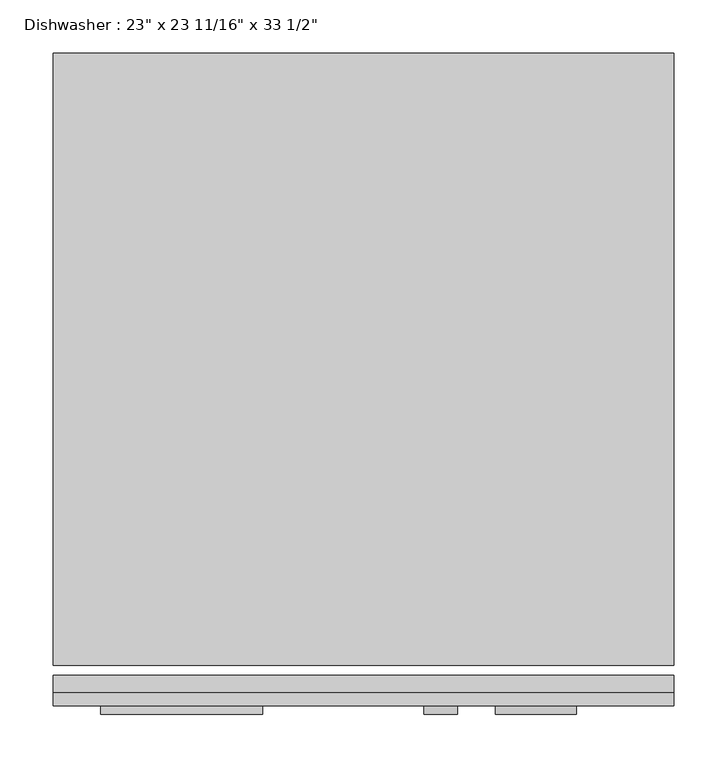
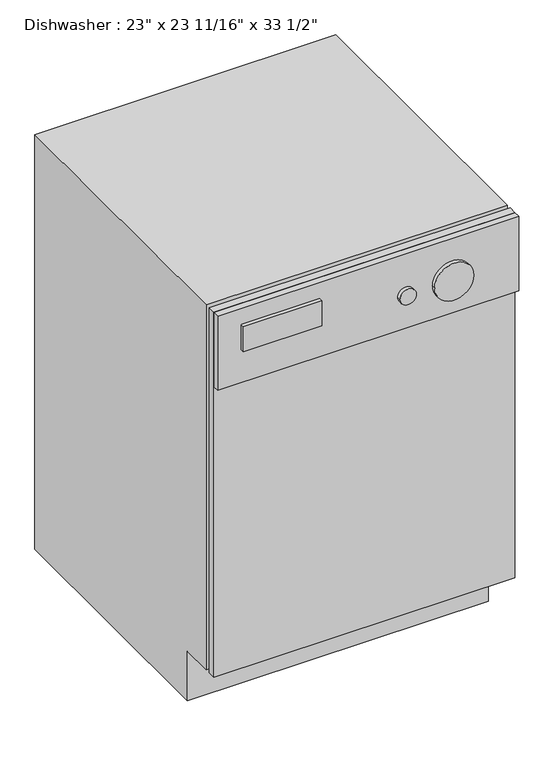
"""IFC4 building model written with IfcOpenShell, lengths in millimetres: proxy geometry."""

from ifc_helpers import new_model, si_unit, point, frame, frame_2d, origin, place, context, project, spatial, polyline, circle_curve, trimmed, segment, composite_curve, outline, extrude, source, transform, mapped, element, save


def proxy_53e5fb40(model_context):
    return source(origin(), model_context, "Body", "SweptSolid", [
        extrude(outline(polyline([(661.7174685, -38.3504352), (77.5174685, -38.3504352), (77.5174685, -22.4754352), (661.7174685, -22.4754352), (661.7174685, -38.3504352)])), frame((0.0, 0.0, 101.6), z_axis=(0.0, 0.0, 1.0), x_axis=(1.0, 0.0, 0.0)), (0.0, 0.0, 1.0), 749.3),
        extrude(outline(polyline([(661.7174685, -38.3504352), (661.7174685, -51.0504352), (77.5174685, -51.0504352), (77.5174685, -38.3504352), (661.7174685, -38.3504352)])), frame((0.0, 0.0, 698.5), z_axis=(0.0, 0.0, 1.0), x_axis=(1.0, 0.0, 0.0)), (0.0, 0.0, 1.0), 152.4),
        extrude(outline(polyline([(563.3120648, 0.0), (50.5495648, 0.0), (50.5495648, 101.6), (-12.9504352, 101.6), (-12.9504352, 850.9), (563.3120648, 850.9), (563.3120648, 0.0)])), frame((77.5174685, 0.0, 0.0), z_axis=(1.0, 0.0, 0.0), x_axis=(0.0, 1.0, 0.0)), (0.0, 0.0, 1.0), 584.2),
        extrude(outline(polyline([(274.9378068, -59.1863727), (122.5378068, -59.1863727), (122.5378068, -51.0504352), (274.9378068, -51.0504352), (274.9378068, -59.1863727)])), frame((0.0, 0.0, 767.3846419), z_axis=(0.0, 0.0, 1.0), x_axis=(1.0, 0.0, 0.0)), (0.0, 0.0, 1.0), 50.8),
        extrude(outline(composite_curve([segment(trimmed(circle_curve(frame_2d((767.3846419, 532.0247133)), 38.1), [point((767.3846419, 493.9247133))], [point((767.3846419, 570.1247133))], False, "CARTESIAN"), True, "CONTINUOUS"), segment(trimmed(circle_curve(frame_2d((767.3846419, 532.0247133)), 38.1), [point((767.3846419, 570.1247133))], [point((767.3846419, 493.9247133))], False, "CARTESIAN"), True, "CONTINUOUS")], self_intersect=False)), frame((0.0, -59.1863727, 0.0), z_axis=(0.0, 1.0, 0.0), x_axis=(0.0, 0.0, 1.0)), (0.0, 0.0, 1.0), 8.1359375),
        extrude(outline(composite_curve([segment(trimmed(circle_curve(frame_2d((767.3846419, 442.495318)), 15.875), [point((767.3846419, 426.620318))], [point((767.3846419, 458.370318))], False, "CARTESIAN"), True, "CONTINUOUS"), segment(trimmed(circle_curve(frame_2d((767.3846419, 442.495318)), 15.875), [point((767.3846419, 458.370318))], [point((767.3846419, 426.620318))], False, "CARTESIAN"), True, "CONTINUOUS")], self_intersect=False)), frame((0.0, -59.1863727, 0.0), z_axis=(0.0, 1.0, 0.0), x_axis=(0.0, 0.0, 1.0)), (0.0, 0.0, 1.0), 8.1359375),
    ])


if __name__ == "__main__":
    model = new_model("IFC4")
    model_context = context("Model", 3, world=origin())
    ifc_project = project(units=[si_unit("LENGTHUNIT", "METRE", prefix="MILLI")], contexts=[model_context])
    site = spatial("IfcSite", under=ifc_project)
    building = spatial("IfcBuilding", under=site)
    placement = place(None, origin())
    proxy_shape = proxy_53e5fb40(model_context)
    element("IfcBuildingElementProxy", 1, Name="Dishwasher : 23\" x 23 11/16\" x 33 1/2\"", ObjectType="Dishwasher : 23\" x 23 11/16\" x 33 1/2\"", at=placement, inside=building, context=model_context, shape_type="MappedRepresentation", body=[
        mapped(proxy_shape, transform((0.0, 0.0, 0.0), x_axis=(1.0, 0.0, 0.0), y_axis=(0.0, 1.0, 0.0), z_axis=(0.0, 0.0, 1.0))),
    ])
    save(model, "model.ifc")

# Revit data of these elements
# Type "Dishwasher : 23\" x 23 11/16\" x 33 1/2\""
#   Label = "DW"
#   Assembly Code = "E1090400"
#   Depth = 1' - 11 11/16"
#   Height = 2' - 9 1/2"
#   Width = 1' - 11"
#   Dishwasher Material = Steel, Paint Finish, Ivory, Glossy
#   Panel Face Material = Plastic, Opaque Black
#   Default Elevation = 0
# Element 1 (IfcBuildingElementProxy, "Dishwasher : 23\" x 23 11/16\" x 33 1/2\"")
#   Materials on its faces: "Steel, Paint Finish, Ivory, Glossy", "Plastic, Opaque Black"
# Materials
#   "Steel, Paint Finish, Ivory, Glossy": class "Metal", colour RGB 247 247 239, transparency 0, Description = "Steel, paint finish, ivory, glossy", Cost = 0
#   "Plastic, Opaque Black": class "Plastic", colour RGB 0 0 0, transparency 0.7, Description = "Plastic, generic, opaque black", Cost = 0
